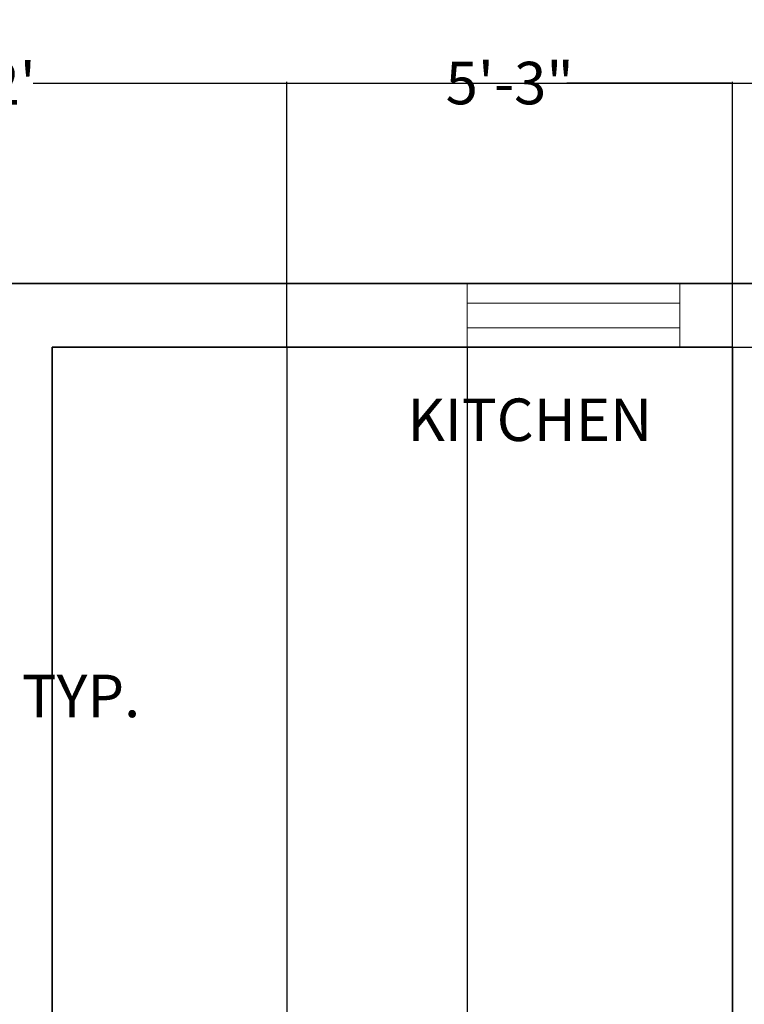
# Model space of a CAD drawing. Units: inches. Extents: x -26 to 575, y -18 to 513.
# Tile 25 of 28: x 274 to 376, y 374 to 513. Entities that reach past the tile are written whole.
import ezdxf

# ---------------------------------------------------------------- set-up
doc = ezdxf.new("R2010")
doc.units = ezdxf.units.IN
doc.header["$MEASUREMENT"] = 0
for name, color, linetype, lineweight in [('A-ANNO-DIMS', 2, 'Continuous', 18), ('A-AREA-IDEN', 7, 'Continuous', 18), ('A-FLOR-CASE', 8, 'Continuous', 18), ('A-GLAZ', 4, 'Continuous', 18), ('A-WALL', 7, 'Continuous', 35)]:
    doc.layers.add(name, color=color, linetype=linetype, lineweight=lineweight)
doc.styles.get("Standard").update_dxf_attribs({"font": 'arial.ttf', "height": 6})
doc.dimstyles.get("Standard").update_dxf_attribs({"dimtxt": 6, "dimasz": 0.18, "dimexe": 0.18, "dimexo": 0.0625, "dimgap": 0.09, "dimtad": 0, "dimtih": 1, "dimtoh": 1, "dimzin": 0, "dimdsep": 46, "dimlunit": 3, "dimtxsty": 'Standard', "dimcen": 0.09, "dimadec": 0, "dimazin": 0, "dimtfac": 1, "dimtofl": 0, "dimtmove": 0, "dimatfit": 3, "dimfxl": 1, "dimtolj": 1, "dimtzin": 0, "dimarcsym": 0})

# ---------------------------------------------------------------- blocks, each defined once
blk = doc.blocks.new('*D1')
at = {"layer": 'A-ANNO-DIMS', "color": 0, "lineweight": -2, "transparency": 16777216}
for p, q in [((18.18, 475.57), (18.18, 503.94)), ((18.36, 503.76), (264.87, 503.76)), ((522, 503.76), (275.48, 503.76)), ((522.18, 475.57), (522.18, 503.94))]:
    blk.add_line(p, q, dxfattribs=at)
at = {"layer": 'A-ANNO-DIMS', "color": 0, "transparency": 16777216}
for points in [[(18.36, 503.79), (18.36, 503.73), (18.18, 503.76)], [(522, 503.79), (522, 503.73), (522.18, 503.76)]]:
    blk.add_solid(points, dxfattribs=at)
at = {"layer": 'Defpoints', "color": 0, "transparency": 16777216}
for p in [(522.18, 503.76), (18.18, 475.51), (522.18, 475.51)]:
    blk.add_point(p, dxfattribs=at)
at = {"layer": 'A-ANNO-DIMS', "color": 0, "transparency": 16777216, "insert": (270.18, 503.76), "char_height": 6, "attachment_point": 5}
blk.add_mtext("\\A1;42'", dxfattribs=at)
blk = doc.blocks.new('WINDOW-30IN')
for p, q in [((30, 9), (0, 9)), ((0, 9), (0, 0)), ((30, 0), (30, 9)), ((30, 6.25), (0, 6.25)), ((30, 0), (30, 4.5)), ((30, 2.75), (0, 2.75)), ((0, 0), (30, 0))]:
    blk.add_line(p, q)
blk = doc.blocks.new('*D12')
at = {"layer": 'A-ANNO-DIMS', "color": 0, "lineweight": -2, "transparency": 16777216}
for p, q in [((143.38, 375.47), (143.38, 359.76)), ((247.35, 375.47), (247.35, 359.76)), ((143.56, 359.94), (247.17, 359.94)), ((247.35, 359.94), (247.53, 359.94))]:
    blk.add_line(p, q, dxfattribs=at)
at = {"layer": 'A-ANNO-DIMS', "color": 0, "transparency": 16777216}
for points in [[(143.56, 359.97), (143.56, 359.91), (143.38, 359.94)], [(247.17, 359.97), (247.17, 359.91), (247.35, 359.94)]]:
    blk.add_solid(points, dxfattribs=at)
at = {"layer": 'Defpoints', "color": 0, "transparency": 16777216}
for p in [(143.38, 375.53), (247.35, 375.53), (247.35, 359.94)]:
    blk.add_point(p, dxfattribs=at)
at = {"layer": 'A-ANNO-DIMS', "color": 0, "transparency": 16777216, "insert": (329.1, 359.94), "char_height": 6, "attachment_point": 5}
blk.add_mtext('\\A1;DOUBLE BED & NIGHTSTANDS 8\'-8" TYP.', dxfattribs=at)
blk = doc.blocks.new('*D13')
at = {"layer": 'A-ANNO-DIMS', "color": 0, "lineweight": -2, "transparency": 16777216}
for p, q in [((247.41, 459.08), (263.12, 459.08)), ((262.94, 458.9), (262.94, 420.5)), ((262.94, 375.71), (262.94, 414.11)), ((247.41, 375.53), (263.12, 375.53))]:
    blk.add_line(p, q, dxfattribs=at)
at = {"layer": 'A-ANNO-DIMS', "color": 0, "transparency": 16777216}
for points in [[(262.91, 458.9), (262.97, 458.9), (262.94, 459.08)], [(262.91, 375.71), (262.97, 375.71), (262.94, 375.53)]]:
    blk.add_solid(points, dxfattribs=at)
at = {"layer": 'Defpoints', "color": 0, "transparency": 16777216}
for p in [(247.35, 459.08), (262.94, 459.08), (247.35, 375.53)]:
    blk.add_point(p, dxfattribs=at)
at = {"layer": 'A-ANNO-DIMS', "color": 0, "transparency": 16777216, "insert": (262.94, 417.3), "char_height": 6, "attachment_point": 5}
blk.add_mtext('\\A1;6\'-11 1/2" TYP.', dxfattribs=at)
blk = doc.blocks.new('*D31')
at = {"layer": 'A-ANNO-DIMS', "color": 0, "lineweight": -2, "transparency": 16777216}
for p, q in [((311.29, 466.45), (311.29, -8.97)), ((336.72, 466.45), (336.72, -8.97)), ((311.47, -8.79), (336.54, -8.79)), ((336.72, -8.79), (336.9, -8.79))]:
    blk.add_line(p, q, dxfattribs=at)
at = {"layer": 'A-ANNO-DIMS', "color": 0, "transparency": 16777216}
for points in [[(311.47, -8.76), (311.47, -8.82), (311.29, -8.79)], [(336.54, -8.76), (336.54, -8.82), (336.72, -8.79)]]:
    blk.add_solid(points, dxfattribs=at)
at = {"layer": 'Defpoints', "color": 0, "transparency": 16777216}
for p in [(311.29, 466.51), (336.72, 466.51), (336.72, -8.79)]:
    blk.add_point(p, dxfattribs=at)
at = {"layer": 'A-ANNO-DIMS', "color": 0, "transparency": 16777216, "insert": (352.01, -8.79), "char_height": 6, "attachment_point": 5}
blk.add_mtext('\\A1;2\'-1 1/2"', dxfattribs=at)
blk = doc.blocks.new('*D32')
at = {"layer": 'A-ANNO-DIMS', "color": 0, "lineweight": -2, "transparency": 16777216}
for p, q in [((374.18, 466.57), (374.18, 503.99)), ((374.36, 503.81), (392.7, 503.81)), ((392.88, 475.57), (392.88, 503.99)), ((392.88, 503.81), (393.06, 503.81))]:
    blk.add_line(p, q, dxfattribs=at)
at = {"layer": 'A-ANNO-DIMS', "color": 0, "transparency": 16777216}
for points in [[(374.36, 503.84), (374.36, 503.78), (374.18, 503.81)], [(392.7, 503.84), (392.7, 503.78), (392.88, 503.81)]]:
    blk.add_solid(points, dxfattribs=at)
at = {"layer": 'Defpoints', "color": 0, "transparency": 16777216}
for p in [(392.88, 503.81), (392.88, 475.51), (374.18, 466.51)]:
    blk.add_point(p, dxfattribs=at)
at = {"layer": 'A-ANNO-DIMS', "color": 0, "transparency": 16777216, "insert": (407.83, 503.81), "char_height": 6, "attachment_point": 5}
blk.add_mtext('\\A1;1\'-6 1/2"', dxfattribs=at)
blk = doc.blocks.new('*D47')
at = {"layer": 'A-ANNO-DIMS', "color": 0, "lineweight": -2, "transparency": 16777216}
for p, q in [((278.18, 466.45), (278.18, -8.97)), ((311.29, 466.45), (311.29, -8.97)), ((278.36, -8.79), (286.62, -8.79)), ((311.11, -8.79), (302.85, -8.79))]:
    blk.add_line(p, q, dxfattribs=at)
at = {"layer": 'A-ANNO-DIMS', "color": 0, "transparency": 16777216}
for points in [[(278.36, -8.76), (278.36, -8.82), (278.18, -8.79)], [(311.11, -8.76), (311.11, -8.82), (311.29, -8.79)]]:
    blk.add_solid(points, dxfattribs=at)
at = {"layer": 'Defpoints', "color": 0, "transparency": 16777216}
for p in [(278.18, 466.51), (311.29, 466.51), (311.29, -8.79)]:
    blk.add_point(p, dxfattribs=at)
at = {"layer": 'A-ANNO-DIMS', "color": 0, "transparency": 16777216, "insert": (294.73, -8.79), "char_height": 6, "attachment_point": 5}
blk.add_mtext('\\A1;2\'-9"', dxfattribs=at)
blk = doc.blocks.new('*D48')
at = {"layer": 'A-ANNO-DIMS', "color": 0, "lineweight": -2, "transparency": 16777216}
for p, q in [((311.29, 466.57), (311.29, 503.99)), ((311.47, 503.81), (334.67, 503.81)), ((374, 503.81), (350.8, 503.81)), ((374.18, 466.57), (374.18, 503.99))]:
    blk.add_line(p, q, dxfattribs=at)
at = {"layer": 'A-ANNO-DIMS', "color": 0, "transparency": 16777216}
for points in [[(311.47, 503.84), (311.47, 503.78), (311.29, 503.81)], [(374, 503.84), (374, 503.78), (374.18, 503.81)]]:
    blk.add_solid(points, dxfattribs=at)
at = {"layer": 'Defpoints', "color": 0, "transparency": 16777216}
for p in [(374.18, 503.81), (311.29, 466.51), (374.18, 466.51)]:
    blk.add_point(p, dxfattribs=at)
at = {"layer": 'A-ANNO-DIMS', "color": 0, "transparency": 16777216, "insert": (342.73, 503.81), "char_height": 6, "attachment_point": 5}
blk.add_mtext('\\A1;5\'-3"', dxfattribs=at)
blk = doc.blocks.new('*D49')
at = {"layer": 'A-ANNO-DIMS', "color": 0, "lineweight": -2, "transparency": 16777216}
for p, q in [((278.24, 466.51), (550.66, 466.51)), ((550.48, 466.33), (550.48, 403.66)), ((550.48, 334.69), (550.48, 397.35)), ((278.24, 334.51), (550.66, 334.51))]:
    blk.add_line(p, q, dxfattribs=at)
at = {"layer": 'A-ANNO-DIMS', "color": 0, "transparency": 16777216}
for points in [[(550.45, 466.33), (550.51, 466.33), (550.48, 466.51)], [(550.45, 334.69), (550.51, 334.69), (550.48, 334.51)]]:
    blk.add_solid(points, dxfattribs=at)
at = {"layer": 'Defpoints', "color": 0, "transparency": 16777216}
for p in [(278.18, 466.51), (550.48, 466.51), (278.18, 334.51)]:
    blk.add_point(p, dxfattribs=at)
at = {"layer": 'A-ANNO-DIMS', "color": 0, "transparency": 16777216, "insert": (550.48, 400.51), "char_height": 6, "attachment_point": 5}
blk.add_mtext('\\A1;11\'-0"', dxfattribs=at)

msp = doc.modelspace()

# ---------------------------------------------------------------- linework, layer by layer
at = {"layer": 'A-FLOR-CASE'}
msp.add_line((311.292, 334.508), (311.292, 466.508), dxfattribs=at)
at = {"layer": 'A-WALL'}
for p, q in [((278.177, 334.508), (278.177, 466.508)), ((374.177, 466.508), (278.177, 466.508)), ((374.177, 334.508), (374.177, 466.508))]:
    msp.add_line(p, q, dxfattribs=at)
msp.add_lwpolyline([(18.177, 19.508), (522.177, 19.508), (522.177, 475.508), (18.177, 475.508)], close=True, dxfattribs=at)

# ---------------------------------------------------------------- block references
at = {"layer": 'A-GLAZ'}
msp.add_blockref('WINDOW-30IN', (336.72, 466.508), dxfattribs=at)

# ---------------------------------------------------------------- texts
at = {"layer": 'A-AREA-IDEN'}
msp.add_text('KITCHEN', height=6, rotation=0.00167, dxfattribs=at).set_placement((328.299, 453.28))

# ---------------------------------------------------------------- dimensions: what is measured, and where the dimension line sits
at = {"layer": 'A-ANNO-DIMS'}
for base, p1, p2, override, picture, middle in [((392.879, 503.808), (374.177, 466.508), (392.879, 475.508), {"dimdec": 1, "dimlfac": 1, "dimrnd": 0, "dimzin": 1, "dimdsep": 46, "dimlunit": 4, "dimfrac": 2}, '*D32', (407.832, 503.808)), ((522.177, 503.757), (18.177, 475.508), (522.177, 475.508), {"dimclrd": 0, "dimclre": 0, "dimclrt": 0}, '*D1', (270.177, 503.757)), ((374.177, 503.808), (311.292, 466.508), (374.177, 466.508), {"dimdec": 1, "dimlfac": 1, "dimrnd": 0, "dimzin": 1, "dimdsep": 46, "dimlunit": 4, "dimfrac": 2}, '*D48', (342.735, 503.808)), ((311.292, -8.792), (278.177, 466.508), (311.292, 466.508), {"dimdec": 1, "dimlfac": 1, "dimrnd": 0, "dimzin": 1, "dimdsep": 46, "dimlunit": 4, "dimfrac": 2}, '*D47', (294.735, -8.792)), ((336.72, -8.792), (311.292, 466.508), (336.72, 466.508), {"dimdec": 1, "dimlfac": 1, "dimrnd": 0, "dimzin": 1, "dimdsep": 46, "dimlunit": 4, "dimfrac": 2}, '*D31', (352.006, -8.792))]:
    dim = msp.add_linear_dim(base=base, p1=p1, p2=p2, dimstyle='Standard', override=override, dxfattribs=at)
    dim.commit()
    dim.dimension.update_dxf_attribs({"geometry": picture, "text_midpoint": middle})
dim = msp.add_linear_dim(base=(550.477, 466.508), p1=(278.177, 334.508), p2=(278.177, 466.508), angle=90, dimstyle='Standard', override={"dimdec": 1, "dimlfac": 1, "dimrnd": 0, "dimzin": 1, "dimdsep": 46, "dimlunit": 4, "dimfrac": 2}, dxfattribs=at)
dim.commit()
dim.dimension.update_dxf_attribs({"geometry": '*D49', "text_midpoint": (550.477, 400.508)})
dim = msp.add_linear_dim(base=(262.943, 459.077), p1=(247.348, 375.531), p2=(247.348, 459.077), angle=90, text='<> TYP.', dimstyle='Standard', override={"dimdec": 1, "dimlfac": 1, "dimrnd": 0, "dimzin": 1, "dimdsep": 46, "dimlunit": 4, "dimfrac": 2}, dxfattribs=at)
dim.commit()
dim.dimension.update_dxf_attribs({"geometry": '*D13', "text_midpoint": (262.943, 417.304)})
dim = msp.add_linear_dim(base=(247.348, 359.935), p1=(143.378, 375.531), p2=(247.348, 375.531), text='DOUBLE BED & NIGHTSTANDS <> TYP.', dimstyle='Standard', override={"dimdec": 1, "dimlfac": 1, "dimrnd": 0, "dimzin": 1, "dimdsep": 46, "dimlunit": 4, "dimfrac": 2}, dxfattribs=at)
dim.commit()
dim.dimension.update_dxf_attribs({"geometry": '*D12', "text_midpoint": (329.097, 359.935)})

doc.saveas('drawing.dxf')
